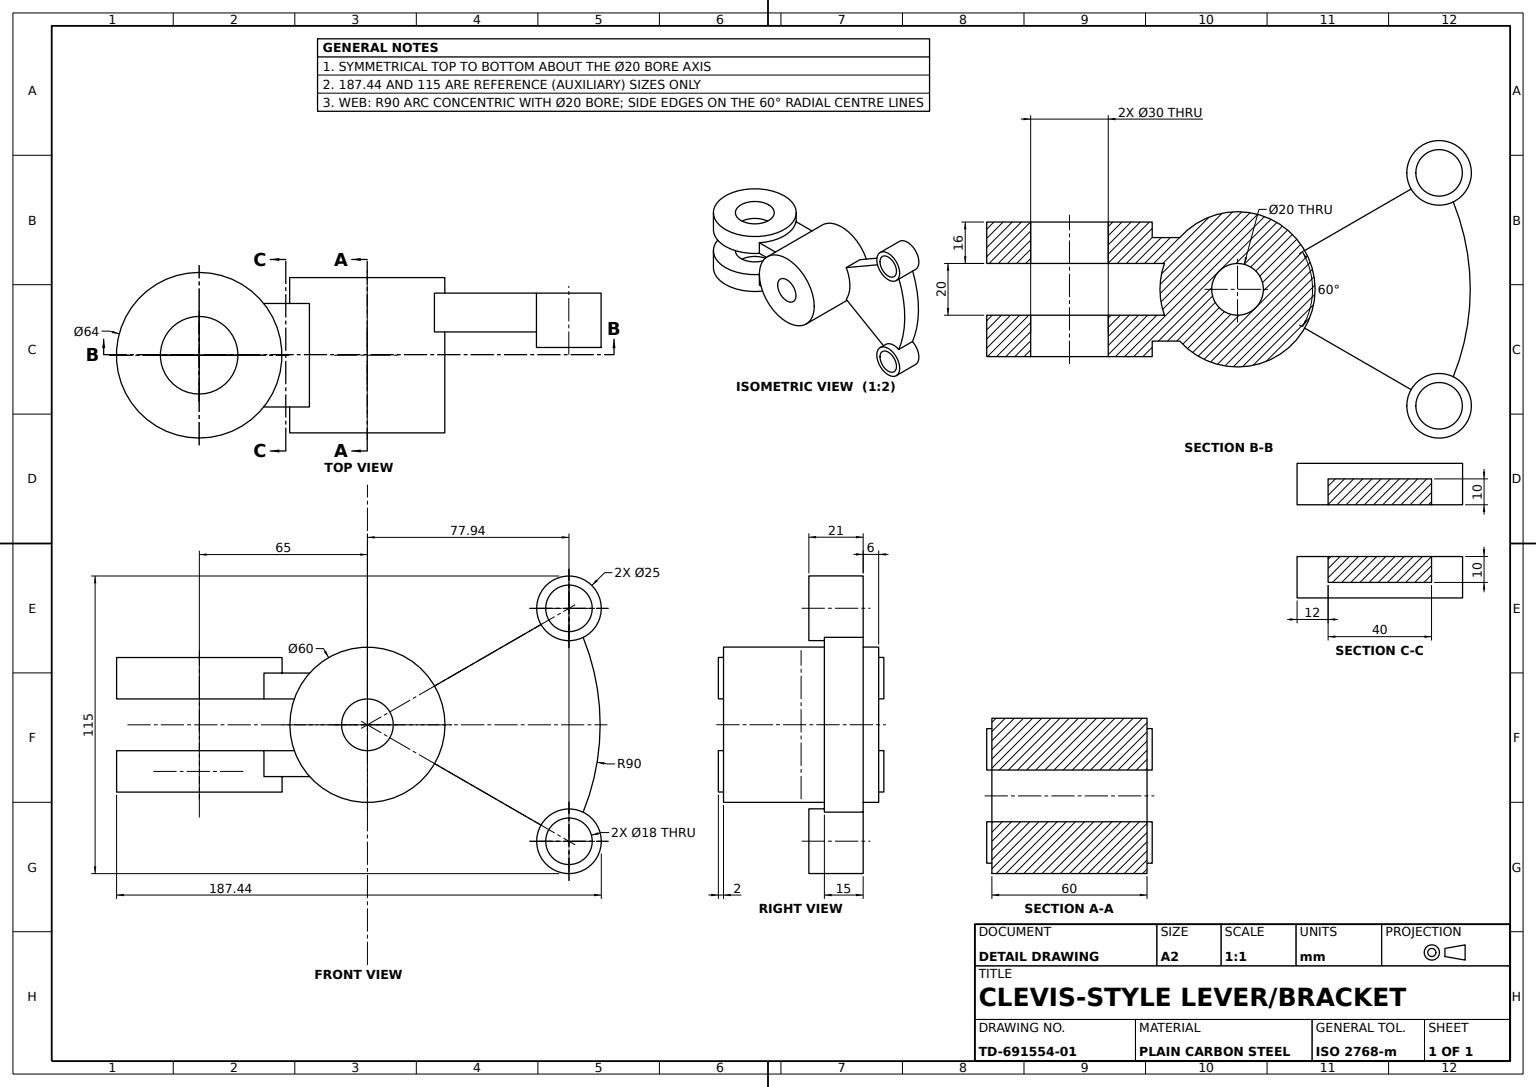
SolidWorks part; units mm, degrees
material "Plain Carbon Steel"
ref_plane "Front Plane" through (0, 0, 0) normal (0, 0, 1) x (1, 0, 0)
ref_plane "Top Plane" through (0, 0, 0) normal (0, 1, 0) x (1, 0, 0)
ref_plane "Right Plane" through (0, 0, 0) normal (1, 0, 0) x (0, 0, -1)
sketch "Hub Sketch" plane through (0, 0, 0) normal (0, 0, 1) x (1, 0, 0)
  circle A0 centre (0, 0) radius 30
  dimension "D1" = 60
extrude "Hub Ø60" add sketch "Hub Sketch" along normal blind 60
ref_plane "Plane2" through (0, 0, 6) normal (0, 0, 1) x (1, 0, 0)
sketch "Mounting Arm Sketch" plane through (0, 0, 6) normal (0, 0, 1) x (1, 0, 0)
  line L0 (0, 0) -> (90, 0) construction
  line L1 (0, 0) -> (77.9423, 45) construction
  line L2 (0, 0) -> (77.9423, -45) construction
  line L3 (0, 0) -> (77.9423, 45)
  line L4 (0, 0) -> (77.9423, -45)
  arc A0 (77.9423, -45) -> (77.9423, 45) centre (0, 0) ccw
  dimension "D1" = 30
  dimension "D3" = 90
  dimension "D2" = 30
extrude "Mounting Arm" add sketch "Mounting Arm Sketch" along normal blind 15
sketch "Upper Lug Boss Sketch" plane through (0, 0, 6) normal (0, 0, 1) x (1, 0, 0)
  circle A0 centre (77.9423, 45) radius 9
  circle A1 centre (77.9423, 45) radius 12.5
  dimension "D1" = 25
  dimension "D2" = 18
extrude "Upper Lug Boss Ø25" add sketch "Upper Lug Boss Sketch" along normal blind 21
sketch "Upper Lug Hole Sketch" plane through (0, 0, 27) normal (0, 0, 1) x (1, 0, 0)
  line L4 (70.1481, 40.5) -> (80.21, 46.3093)
  line L5 (80.21, 46.3093) -> (84.5153, 38.8522)
  circle A2 centre (77.9423, 45) radius 9 construction
  arc A3 (70.1481, 40.5) -> (84.5153, 38.8522) centre (77.9423, 45) ccw
  circle A4 centre (77.9423, 45) radius 12.5 construction
  dimension "D1" = 2.2677
extrude "Upper Lug Hole" cut sketch "Upper Lug Hole Sketch" against normal through all
ref_plane "Plane4" through (0, 10, 0) normal (0, 1, 0) x (1, 0, 0)
sketch "Clevis Arm Sketch" plane through (0, 10, 0) normal (0, 1, 0) x (1, 0, 0)
  line L0 (0, -30) -> (-80, -30) construction
  line L1 (-29.7438, -10) -> (-22.0435, -10)
  line L2 (-22.0435, -10) -> (-22.0435, -50)
  line L3 (-80, -20) -> (-80, -10)
  line L4 (-80, -10) -> (-29.7438, -10)
  line L5 (-80, -20) -> (-65, -20)
  line L6 (-65, -20) -> (-65, -40)
  line L7 (-65, -40) -> (-80, -40)
  line L8 (-80, -40) -> (-80, -50)
  line L9 (-80, -50) -> (-30, -50)
  line L10 (-30, 0) -> (-30, -60) construction
  line L11 (-22.0435, -50) -> (-30, -50)
  dimension "D1" = 30
  dimension "D2" = 40
  dimension "D3" = 10
  dimension "D4" = 10
  dimension "D5" = 15
  dimension "D6" = 50
  dimension "D7" = 7.9565
  dimension "D8" = 50.2562
extrude "Clevis Arm" add sketch "Clevis Arm Sketch" along normal blind 10
ref_plane "Plane5" through (0, 0, 0) normal (0, 1, 0) x (1, 0, 0)
ref_plane "Plane6" through (0, 0, 0) normal (0, 1, 0) x (1, 0, 0)
mirror "Clevis Arm Mirror" about plane through (0, 0, 0) normal (0, 1, 0) of "Clevis Arm"
sketch "Clevis Eye Boss Sketch" plane through (0, 10, 0) normal (0, 1, 0) x (1, 0, 0)
  line L0 (-65, -20) -> (-65, -40) construction
  circle A0 centre (-65, -30) radius 32
  circle A1 centre (-65, -30) radius 15
  dimension "D1" = 30
  dimension "D2" = 64
extrude "Clevis Eye Boss" add sketch "Clevis Eye Boss Sketch" along normal blind 16
mirror "Clevis Eye Boss Mirror" about plane through (0, 0, 0) normal (0, 1, 0) of "Clevis Eye Boss"
sketch "Clevis Eye Hole Sketch" plane through (0, 26, 0) normal (0, 1, 0) x (1, 0, 0)
  line L0 (-65, -20) -> (-65, -40) construction
  circle A0 centre (-65, -30) radius 15
  dimension "D1" = 30
extrude "Clevis Eye Hole" cut sketch "Clevis Eye Hole Sketch" against normal through all
ref_plane "Plane8" through (0, 0, 6) normal (0, 0, 1) x (1, 0, 0)
sketch "Hub Bore Sketch" plane through (0, 0, 60) normal (0, 0, 1) x (1, 0, 0)
  circle A0 centre (0, 0) radius 10
  dimension "D1" = 20
extrude "Hub Bore Ø20" cut sketch "Hub Bore Sketch" against normal through all
ref_plane "Plane9" through (0, 0, 6) normal (0, 0, 1) x (1, 0, 0)
sketch "Lower Lug Boss Sketch" plane through (0, 0, 6) normal (0, 0, 1) x (1, 0, 0)
  circle A0 centre (77.9423, -45) radius 9
  circle A1 centre (77.9423, -45) radius 12.5
  dimension "D1" = 18
  dimension "D2" = 25
extrude "Lower Lug Boss" add sketch "Lower Lug Boss Sketch" along normal blind 21
sketch "Lower Lug Hole Sketch" plane through (0, 0, 21) normal (0, 0, 1) x (1, 0, 0)
  line L0 (77.9423, -45) -> (70.1481, -40.5)
  arc A0 (82.0469, -36.9905) -> (77.9423, -45) centre (0, 0) cw
  arc A2 (82.0469, -36.9905) -> (70.1481, -40.5) centre (77.9423, -45) ccw
extrude "Lower Lug Hole" cut sketch "Lower Lug Hole Sketch" against normal through all
